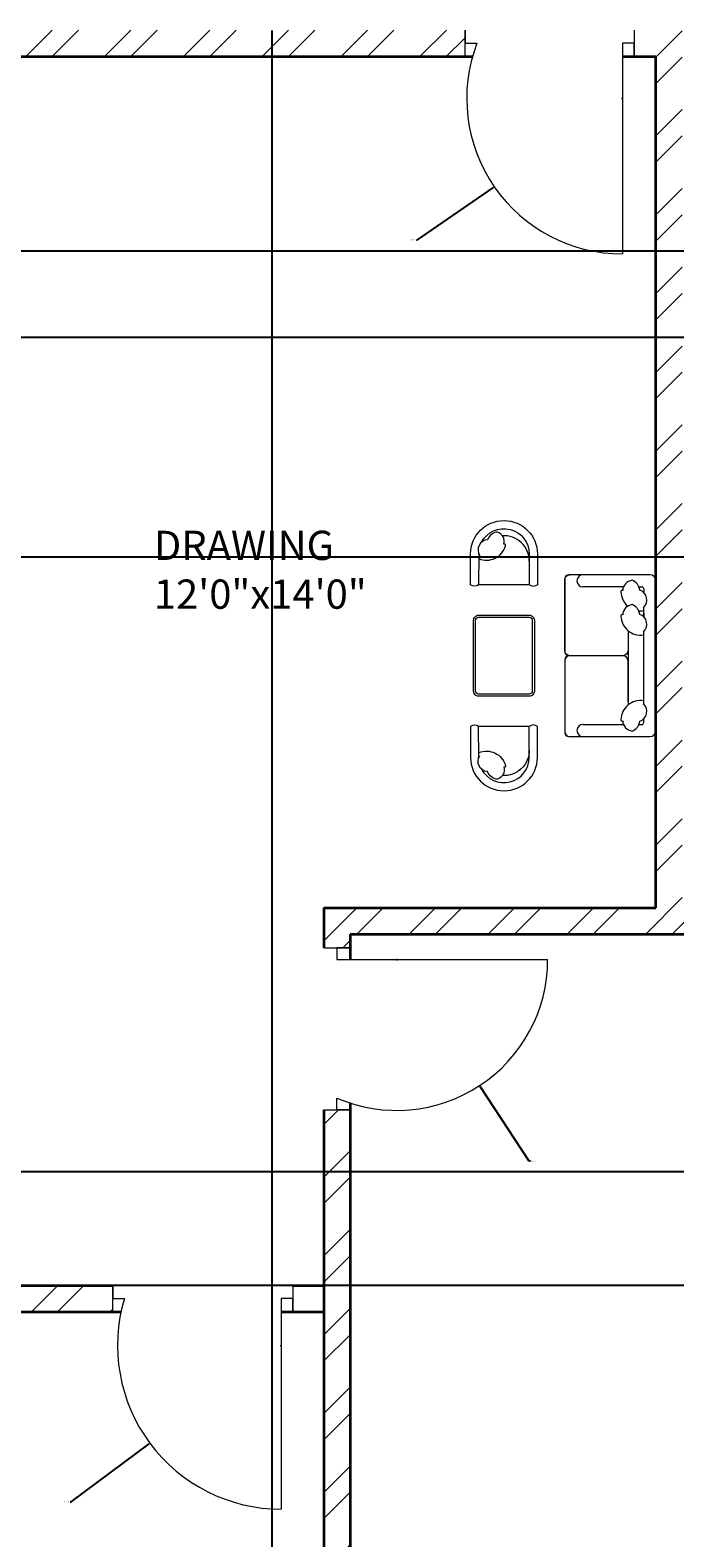
# Model space of a CAD drawing. Units: inches. Extents: x 2008 to 2657, y 1077 to 2165.
# Tile 4 of 16: x 2196 to 2306, y 1309 to 1567. Entities that reach past the tile are written whole.
import ezdxf

# ---------------------------------------------------------------- set-up
doc = ezdxf.new("R2010")
doc.units = ezdxf.units.IN
for name, color, linetype, lineweight in [('A-ANNO-DIMS', 2, 'Continuous', 18), ('A-AREA-IDEN', 4, 'Continuous', 18), ('A-DOOR', 11, 'Continuous', 18), ('A-FURN', 8, 'Continuous', 13), ('A-WALL', 7, 'Continuous', 35)]:
    doc.layers.add(name, color=color, linetype=linetype, lineweight=lineweight)
doc.layers.add('A-WALL-PATT', color=30, linetype='Continuous', lineweight=13, true_color=0xf8991e)
doc.styles.get("Standard").update_dxf_attribs({"font": 'arial.ttf'})
doc.dimstyles.get("Standard").update_dxf_attribs({"dimtxt": 0.18, "dimasz": 0.18, "dimexe": 0.18, "dimexo": 0.0625, "dimgap": 0.09, "dimtad": 0, "dimtih": 1, "dimtoh": 1, "dimdec": 4, "dimzin": 0, "dimdsep": 46, "dimtxsty": 'Standard', "dimcen": 0.09, "dimadec": 0, "dimazin": 0, "dimtfac": 1, "dimtdec": 4, "dimtofl": 0, "dimtmove": 0, "dimatfit": 3, "dimfxl": 1, "dimtolj": 1, "dimtzin": 0, "dimarcsym": 0})

# ---------------------------------------------------------------- blocks, each defined once
blk = doc.blocks.new('A$C1352')
at = {"color": 0}
for points in [[(0.003, 0.053), (0.003, 0.553, -0.414214), (0.053, 0.603), (0.753, 0.603, -0.414214), (0.803, 0.553), (0.803, 0.053, -0.414214), (0.753, 0.003), (0.053, 0.003, -0.414214)], [(0.023, 0.053), (0.023, 0.553, -0.414214), (0.053, 0.583), (0.753, 0.583, -0.414214), (0.783, 0.553), (0.783, 0.053, -0.414214), (0.753, 0.023), (0.053, 0.023, -0.414214)]]:
    blk.add_lwpolyline(points, format="xyb", close=True, dxfattribs=at)
blk = doc.blocks.new('LOUNGE-CHAIR')
blk.add_line((1.39, 5.54), (1.38, 0.26))
at = {"ltscale": 0.03}
blk.add_lwpolyline([(1.38, 0.26, -0.369229), (0, 0.27), (0, 5.54, -1), (11.42, 5.53), (11.42, 0.25, -0.369229), (10.03, 0.26)], format="xyb", close=True, dxfattribs=at)
blk.add_lwpolyline([(1.88, 7.54, -0.785087), (10.04, 5.53), (10.03, 0.26)], format="xyb")
for centre, radius, start, end in [((3.01, 6.23), 1.73, 92.9922, 214.1401), ((4.77, 7.34), 1.95, 94.9999, 161.3534), ((3.98, 7.61), 1.78, 346.6403, 69.4695), ((5.71, 4.32), 4.33, 359.9461, 93.658), ((5.71, 5.54), 4.33, 178.8536, 179.9461), ((2.75, 7.82), 3.35, 247.0143, 344.2857), ((5.79, 7.01), 0.207, 330.6238, 113.7423)]:
    blk.add_arc(centre, radius, start, end)
blk = doc.blocks.new('*D31')
at = {"layer": 'A-ANNO-DIMS', "color": 0, "lineweight": -2, "transparency": 16777216}
for p, q in [((2076.26, 1562.18), (2076.26, 1140.44)), ((2576.76, 1188.61), (2576.76, 1140.44)), ((2076.44, 1140.62), (2326.12, 1140.62)), ((2576.58, 1140.62), (2326.91, 1140.62))]:
    blk.add_line(p, q, dxfattribs=at)
at = {"layer": 'A-ANNO-DIMS', "color": 0, "transparency": 16777216}
for points in [[(2076.44, 1140.65), (2076.44, 1140.59), (2076.26, 1140.62)], [(2576.58, 1140.65), (2576.58, 1140.59), (2576.76, 1140.62)]]:
    blk.add_solid(points, dxfattribs=at)
at = {"layer": 'Defpoints', "color": 0, "transparency": 16777216}
for p in [(2076.26, 1562.24), (2576.76, 1188.67), (2576.76, 1140.62)]:
    blk.add_point(p, dxfattribs=at)
at = {"layer": 'A-ANNO-DIMS', "color": 0, "transparency": 16777216, "insert": (2326.51, 1140.62), "char_height": 0.18, "attachment_point": 5}
blk.add_mtext('\\A1;500.5', dxfattribs=at)
blk = doc.blocks.new('*D53')
at = {"layer": 'A-ANNO-DIMS', "color": 0, "lineweight": -2, "transparency": 16777216}
for p, q in [((2406.7, 1613.17), (2028.03, 1613.17)), ((2028.21, 1612.99), (2028.21, 1545.11)), ((2028.21, 1476.85), (2028.21, 1544.74)), ((2406.7, 1476.67), (2028.03, 1476.67))]:
    blk.add_line(p, q, dxfattribs=at)
at = {"layer": 'A-ANNO-DIMS', "color": 0, "transparency": 16777216}
for points in [[(2028.18, 1612.99), (2028.24, 1612.99), (2028.21, 1613.17)], [(2028.18, 1476.85), (2028.24, 1476.85), (2028.21, 1476.67)]]:
    blk.add_solid(points, dxfattribs=at)
at = {"layer": 'Defpoints', "color": 0, "transparency": 16777216}
for p in [(2406.76, 1613.17), (2028.21, 1476.67), (2406.76, 1476.67)]:
    blk.add_point(p, dxfattribs=at)
at = {"layer": 'A-ANNO-DIMS', "color": 0, "transparency": 16777216, "insert": (2028.21, 1544.92), "char_height": 0.18, "attachment_point": 5}
blk.add_mtext('\\A1;136.5', dxfattribs=at)
blk = doc.blocks.new('*D62')
at = {"layer": 'A-ANNO-DIMS', "color": 0, "lineweight": -2, "transparency": 16777216}
for p, q in [((2117.38, 1566.68), (2117.38, 1140.44)), ((2237.38, 1566.68), (2237.38, 1140.44)), ((2117.56, 1140.62), (2177.1, 1140.62)), ((2237.2, 1140.62), (2177.66, 1140.62))]:
    blk.add_line(p, q, dxfattribs=at)
at = {"layer": 'A-ANNO-DIMS', "color": 0, "transparency": 16777216}
for points in [[(2117.56, 1140.65), (2117.56, 1140.59), (2117.38, 1140.62)], [(2237.2, 1140.65), (2237.2, 1140.59), (2237.38, 1140.62)]]:
    blk.add_solid(points, dxfattribs=at)
at = {"layer": 'Defpoints', "color": 0, "transparency": 16777216}
for p in [(2117.38, 1566.74), (2237.38, 1566.74), (2237.38, 1140.62)]:
    blk.add_point(p, dxfattribs=at)
at = {"layer": 'A-ANNO-DIMS', "color": 0, "transparency": 16777216, "insert": (2177.38, 1140.62), "char_height": 0.18, "attachment_point": 5}
blk.add_mtext('\\A1;120', dxfattribs=at)
blk = doc.blocks.new('*D68')
at = {"layer": 'A-ANNO-DIMS', "color": 0, "lineweight": -2, "transparency": 16777216}
for p, q in [((2572.2, 1371.57), (2028.03, 1371.57)), ((2028.21, 1371.39), (2028.21, 1362.05)), ((2028.21, 1352.35), (2028.21, 1361.69)), ((2572.2, 1352.17), (2028.03, 1352.17))]:
    blk.add_line(p, q, dxfattribs=at)
at = {"layer": 'A-ANNO-DIMS', "color": 0, "transparency": 16777216}
for points in [[(2028.18, 1371.39), (2028.24, 1371.39), (2028.21, 1371.57)], [(2028.18, 1352.35), (2028.24, 1352.35), (2028.21, 1352.17)]]:
    blk.add_solid(points, dxfattribs=at)
at = {"layer": 'Defpoints', "color": 0, "transparency": 16777216}
for p in [(2028.21, 1371.57), (2572.26, 1371.57), (2572.26, 1352.17)]:
    blk.add_point(p, dxfattribs=at)
at = {"layer": 'A-ANNO-DIMS', "color": 0, "transparency": 16777216, "insert": (2028.21, 1361.87), "char_height": 0.18, "attachment_point": 5}
blk.add_mtext('\\A1;19.394', dxfattribs=at)
blk = doc.blocks.new('*D69')
at = {"layer": 'A-ANNO-DIMS', "color": 0, "lineweight": -2, "transparency": 16777216}
for p, q in [((2109.32, 1529), (2624.99, 1529)), ((2624.81, 1528.82), (2624.81, 1521.8)), ((2624.81, 1514.42), (2624.81, 1521.44)), ((2109.32, 1514.24), (2624.99, 1514.24))]:
    blk.add_line(p, q, dxfattribs=at)
at = {"layer": 'A-ANNO-DIMS', "color": 0, "transparency": 16777216}
for points in [[(2624.78, 1528.82), (2624.84, 1528.82), (2624.81, 1529)], [(2624.78, 1514.42), (2624.84, 1514.42), (2624.81, 1514.24)]]:
    blk.add_solid(points, dxfattribs=at)
at = {"layer": 'Defpoints', "color": 0, "transparency": 16777216}
for p in [(2109.26, 1529), (2624.81, 1529), (2109.26, 1514.24)]:
    blk.add_point(p, dxfattribs=at)
at = {"layer": 'A-ANNO-DIMS', "color": 0, "transparency": 16777216, "insert": (2624.81, 1521.62), "char_height": 0.18, "attachment_point": 5}
blk.add_mtext('\\A1;14.756', dxfattribs=at)
blk = doc.blocks.new('*D75')
at = {"layer": 'A-ANNO-DIMS', "color": 0, "lineweight": -2, "transparency": 16777216}
for p, q in [((2238.91, 1341.89), (2239.09, 1341.89)), ((2239, 1341.8), (2239, 1341.98)), ((2203.1, 1315.18), (2216.42, 1325.09)), ((2202.92, 1315.18), (2203.1, 1315.18))]:
    blk.add_line(p, q, dxfattribs=at)
at = {"layer": 'A-ANNO-DIMS', "color": 0, "transparency": 16777216}
blk.add_solid([(2216.4, 1325.11), (2216.43, 1325.06), (2216.56, 1325.2)], dxfattribs=at)
at = {"layer": 'Defpoints', "color": 0, "transparency": 16777216}
for p in [(2239, 1341.89), (2216.56, 1325.2)]:
    blk.add_point(p, dxfattribs=at)
at = {"layer": 'A-ANNO-DIMS', "color": 0, "transparency": 16777216, "insert": (2202.37, 1315.18), "char_height": 0.18, "attachment_point": 5}
blk.add_mtext('\\A1;R27.965', dxfattribs=at)
blk = doc.blocks.new('*D78')
at = {"layer": 'A-ANNO-DIMS', "color": 0, "lineweight": -2, "transparency": 16777216}
for p, q in [((2297.18, 1555.08), (2297.36, 1555.08)), ((2297.27, 1554.99), (2297.27, 1555.17)), ((2262.27, 1530.9), (2275.25, 1539.87)), ((2262.09, 1530.9), (2262.27, 1530.9))]:
    blk.add_line(p, q, dxfattribs=at)
at = {"layer": 'A-ANNO-DIMS', "color": 0, "transparency": 16777216}
blk.add_solid([(2275.23, 1539.89), (2275.26, 1539.84), (2275.39, 1539.97)], dxfattribs=at)
at = {"layer": 'Defpoints', "color": 0, "transparency": 16777216}
for p in [(2297.27, 1555.08), (2275.39, 1539.97)]:
    blk.add_point(p, dxfattribs=at)
at = {"layer": 'A-ANNO-DIMS', "color": 0, "transparency": 16777216, "insert": (2261.61, 1530.9), "char_height": 0.18, "attachment_point": 5}
blk.add_mtext('\\A1;R26.59', dxfattribs=at)
blk = doc.blocks.new('*D80')
at = {"layer": 'A-ANNO-DIMS', "color": 0, "lineweight": -2, "transparency": 16777216}
for p, q in [((2258.65, 1407.86), (2258.83, 1407.86)), ((2258.74, 1407.77), (2258.74, 1407.95)), ((2281.38, 1373.4), (2272.99, 1386.17)), ((2281.56, 1373.4), (2281.38, 1373.4))]:
    blk.add_line(p, q, dxfattribs=at)
at = {"layer": 'A-ANNO-DIMS', "color": 0, "transparency": 16777216}
blk.add_solid([(2273.02, 1386.19), (2272.97, 1386.16), (2272.89, 1386.32)], dxfattribs=at)
at = {"layer": 'Defpoints', "color": 0, "transparency": 16777216}
for p in [(2258.74, 1407.86), (2272.89, 1386.32)]:
    blk.add_point(p, dxfattribs=at)
at = {"layer": 'A-ANNO-DIMS', "color": 0, "transparency": 16777216, "insert": (2282.04, 1373.4), "char_height": 0.18, "attachment_point": 5}
blk.add_mtext('\\A1;R25.77', dxfattribs=at)

msp = doc.modelspace()

# ---------------------------------------------------------------- hatches: boundary and pattern name
at = {"layer": 'A-WALL-PATT'}
h = msp.add_hatch(dxfattribs=at)
h.set_pattern_fill('ANSI32', color=256)
h.paths.add_polyline_path([(2109.2619, 2094.6743), (2104.7619, 2094.6743), (2104.7619, 2072.1743), (2104.7619, 2021.6151), (2109.2619, 2021.6151), (2109.2619, 2055.6743), (2126.1387, 2055.6743), (2126.1387, 2057.9243), (2126.1387, 2060.1743), (2109.2619, 2060.1743)])
h.paths.add_polyline_path([(2223.2494, 2057.9243), (2223.2494, 2060.1743), (2186.1387, 2060.1743), (2186.1387, 2055.6743), (2223.2494, 2055.6743)])
h.paths.add_polyline_path([(2250.7619, 2072.1743), (2250.7619, 2090.1743), (2250.7619, 2094.6743), (2246.2619, 2094.6743), (2246.2619, 2060.1743), (2242.7242, 2060.1743), (2242.7242, 2055.6743), (2246.2619, 2055.6743), (2246.2619, 1899.6743), (2242.7458, 1899.6743), (2242.7458, 1897.4243), (2242.7458, 1895.1743), (2246.2619, 1895.1743), (2246.2619, 1878.8745), (2248.5119, 1878.8745), (2250.7619, 1878.8745), (2250.7619, 1991.1743), (2250.7619, 2025.6743), (2257.6798, 2025.6743), (2257.6798, 2027.9243), (2257.6798, 2030.1743), (2250.7619, 2030.1743)])
h.paths.add_polyline_path([(2411.2619, 2031.6743), (2409.0119, 2031.6743), (2406.7619, 2031.6743), (2406.7619, 2030.1743), (2322.7619, 2030.1743), (2322.7619, 2053.3443), (2318.2619, 2053.3443), (2318.2619, 2030.1743), (2305.6798, 2030.1743), (2305.6798, 2025.6743), (2318.2619, 2025.6743), (2322.7619, 2025.6743), (2406.7619, 2025.6743), (2406.7619, 1995.6743), (2406.7619, 1847.2677), (2250.7619, 1847.2677), (2250.7619, 1850.9902), (2248.5119, 1850.9902), (2246.2619, 1850.9902), (2246.2619, 1847.1743), (2246.2619, 1842.7677), (2303.0015, 1842.7677), (2303.0015, 1667.2413), (2298.4208, 1667.2413), (2298.4208, 1662.7413), (2303.0015, 1662.7413), (2303.0015, 1649.8758), (2307.5015, 1649.8758), (2307.5015, 1842.7677), (2406.7619, 1842.7677), (2411.2619, 1842.7677), (2411.2619, 1878.6743), (2415.8196, 1878.6743), (2415.8196, 1880.9243), (2415.8196, 1883.1743), (2411.2619, 1883.1743)])
h.paths.add_polyline_path([(2411.2619, 2094.6743), (2406.7619, 2094.6743), (2318.2619, 2094.6743), (2318.2619, 2077.3443), (2322.7619, 2077.3443), (2322.7619, 2090.1743), (2406.7619, 2090.1743), (2406.7619, 2072.1743), (2406.7619, 2067.6743), (2406.7619, 2052.7524), (2411.2619, 2052.7524), (2411.2619, 2055.6743), (2414.9888, 2055.6743), (2414.9888, 2057.9243), (2414.9888, 2060.1743), (2411.2619, 2060.1743), (2411.2619, 2072.1743)])
h.paths.add_polyline_path([(2576.7619, 2072.1743), (2576.7619, 2094.6743), (2572.2619, 2094.6743), (2572.2619, 2060.1743), (2525.8113, 2060.1743), (2525.8113, 2055.6743), (2572.2619, 2055.6743), (2572.2619, 1994.289), (2576.7619, 1994.289)])
h.paths.add_polyline_path([(2465.8113, 2060.1743), (2436.2802, 2060.1743), (2436.2802, 2055.6743), (2465.8113, 2055.6743), (2465.8113, 2057.9243)])
h.paths.add_polyline_path([(2576.7619, 1934.289), (2574.5119, 1934.289), (2572.2619, 1934.289), (2572.2619, 1883.1743), (2447.7027, 1883.1743), (2447.7027, 1878.6743), (2459.7619, 1878.6743), (2459.7619, 1830.4982), (2464.2619, 1830.4982), (2464.2619, 1878.6743), (2572.2619, 1878.6743), (2572.2619, 1868.4883), (2576.7619, 1868.4883)])
h.paths.add_polyline_path([(2576.7619, 1832.4883), (2572.2619, 1832.4883), (2572.2619, 1806.6743), (2464.2619, 1806.6743), (2464.2619, 1809.6629), (2459.7619, 1809.6629), (2459.7619, 1802.1743), (2483.7619, 1802.1743), (2483.7619, 1778.1743), (2488.2619, 1778.1743), (2488.2619, 1802.1743), (2572.2619, 1802.1743), (2572.2619, 1793.6101), (2576.7619, 1793.6101)])
h.paths.add_polyline_path([(2576.7619, 1769.6101), (2572.2619, 1769.6101), (2572.2619, 1754.1743), (2488.2619, 1754.1743), (2488.2619, 1757.2675), (2486.0119, 1757.2675), (2483.7619, 1757.2675), (2483.7619, 1754.1743), (2447.4528, 1754.1743), (2447.4528, 1749.6743), (2483.7619, 1749.6743), (2572.2619, 1749.6743), (2572.2619, 1715.1837), (2576.7619, 1715.1837)])
h.paths.add_polyline_path([(2576.7619, 1655.1837), (2572.2619, 1655.1837), (2572.2619, 1617.6743), (2411.2619, 1617.6743), (2411.2619, 1749.6743), (2414.2827, 1749.6743), (2414.2827, 1754.1743), (2406.7619, 1754.1743), (2406.7619, 1749.6743), (2406.7619, 1617.6743), (2307.5015, 1617.6743), (2307.5015, 1621.0007), (2305.2515, 1621.0007), (2303.0015, 1621.0007), (2303.0015, 1609.6944), (2307.5015, 1609.6944), (2307.5015, 1613.1743), (2406.7619, 1613.1743), (2406.7619, 1476.6743), (2415.532, 1476.6743), (2415.532, 1478.9243), (2415.532, 1481.1743), (2411.2619, 1481.1743), (2411.2619, 1613.1743), (2572.2619, 1613.1743), (2572.2619, 1584.6086), (2576.7619, 1584.6086)])
h.paths.add_polyline_path([(2576.7619, 1524.6086), (2572.2619, 1524.6086), (2572.2619, 1481.1743), (2483.7619, 1481.1743), (2447.5119, 1481.1743), (2447.5119, 1476.6743), (2483.7619, 1476.6743), (2483.7619, 1473.5051), (2488.2619, 1473.5051), (2488.2619, 1476.6743), (2572.2619, 1476.6743), (2572.2619, 1469.5488), (2576.7619, 1469.5488)])
h.paths.add_polyline_path([(2576.7619, 1445.5488), (2572.2619, 1445.5488), (2572.2619, 1428.6743), (2488.2619, 1428.6743), (2488.2619, 1455.6743), (2486.0119, 1455.6743), (2483.7619, 1455.6743), (2483.7619, 1428.6743), (2459.7619, 1428.6743), (2459.7619, 1422.1519), (2464.2619, 1422.1519), (2464.2619, 1424.1743), (2572.2619, 1424.1743), (2572.2619, 1407.5685), (2576.7619, 1407.5685)])
h.paths.add_polyline_path([(2576.7619, 1371.5685), (2572.2619, 1371.5685), (2572.2619, 1352.1743), (2464.2619, 1352.1743), (2464.2619, 1403.1384), (2462.0119, 1403.1384), (2459.7619, 1403.1384), (2459.7619, 1352.1743), (2446.3194, 1352.1743), (2446.3194, 1347.6743), (2572.2619, 1347.6743), (2572.2619, 1321.0291), (2576.7619, 1321.0291)])
h.paths.add_polyline_path([(2462.703, 1227.6743), (2436.0298, 1227.6743), (2436.0298, 1225.4243), (2436.0298, 1223.1743), (2462.703, 1223.1743), (2462.703, 1225.4243)])
h.paths.add_polyline_path([(2576.7619, 1261.0291), (2574.5119, 1261.0291), (2572.2619, 1261.0291), (2572.2619, 1227.6743), (2522.703, 1227.6743), (2522.703, 1223.1743), (2572.2619, 1223.1743), (2572.2619, 1188.6743), (2576.7619, 1188.6743), (2576.7619, 1193.1743), (2576.7619, 1223.1743)])
h.paths.add_polyline_path([(2414.2823, 1227.6743), (2411.2619, 1227.6743), (2411.2619, 1267.1779), (2409.0119, 1267.1779), (2406.7619, 1267.1779), (2406.7619, 1227.6743), (2322.7619, 1227.6743), (2322.7619, 1244.3623), (2318.2619, 1244.3623), (2318.2619, 1223.1743), (2406.7619, 1223.1743), (2406.7619, 1193.1743), (2406.7619, 1188.6743), (2411.2619, 1188.6743), (2411.2619, 1193.1743), (2411.2619, 1223.1743), (2414.2823, 1223.1743)])
h.paths.add_polyline_path([(2411.2619, 1347.6743), (2414.702, 1347.6743), (2414.702, 1349.9243), (2414.702, 1352.1743), (2411.2619, 1352.1743), (2411.2619, 1416.7413), (2307.5015, 1416.7413), (2307.5015, 1579.8489), (2305.2515, 1579.8489), (2303.0015, 1579.8489), (2303.0015, 1566.7413), (2299.2719, 1566.7413), (2299.2719, 1562.2413), (2303.0015, 1562.2413), (2303.0015, 1416.7413), (2246.2619, 1416.7413), (2246.2619, 1409.8616), (2250.7619, 1409.8616), (2250.7619, 1412.2413), (2406.7619, 1412.2413), (2406.7619, 1292.1743), (2304.9703, 1292.1743), (2304.9703, 1287.6743), (2318.2619, 1287.6743), (2318.2619, 1268.3623), (2322.7619, 1268.3623), (2322.7619, 1287.6743), (2406.7619, 1287.6743), (2406.7619, 1285.4748), (2411.2619, 1285.4748)])
h.paths.add_polyline_path([(2109.2619, 1262.7482), (2104.7619, 1262.7482), (2104.7619, 1223.1743), (2104.7619, 1193.1743), (2104.7619, 1188.6743), (2109.2619, 1188.6743), (2109.2619, 1223.1743), (2126.7928, 1223.1743), (2126.7928, 1225.4243), (2126.7928, 1227.6743), (2109.2619, 1227.6743)])
h.paths.add_polyline_path([(2222.3268, 1227.6743), (2186.7928, 1227.6743), (2186.7928, 1223.1743), (2222.3268, 1223.1743)])
h.paths.add_polyline_path([(2250.7619, 1287.6743), (2256.9703, 1287.6743), (2256.9703, 1289.9243), (2256.9703, 1292.1743), (2250.7619, 1292.1743), (2250.7619, 1382.2078), (2248.5119, 1382.2078), (2246.2619, 1382.2078), (2246.2619, 1347.6743), (2246.2619, 1227.6743), (2242.6068, 1227.6743), (2242.6068, 1223.1743), (2246.2619, 1223.1743), (2246.2619, 1188.6743), (2250.7619, 1188.6743), (2250.7619, 1193.1743), (2250.7619, 1227.6743)])
h.paths.add_polyline_path([(2133.2619, 1349.9243), (2133.2619, 1352.1743), (2109.2619, 1352.1743), (2109.2619, 1375.2826), (2104.7619, 1375.2826), (2104.7619, 1322.7482), (2109.2619, 1322.7482), (2109.2619, 1347.6743), (2133.2619, 1347.6743)])
h.paths.add_polyline_path([(2210.2105, 1352.1743), (2161.7619, 1352.1743), (2161.7619, 1412.2413), (2185.7619, 1412.2413), (2185.7619, 1420.1851), (2183.5119, 1420.1851), (2181.2619, 1420.1851), (2181.2619, 1416.7413), (2109.2619, 1416.7413), (2109.2619, 1452.4006), (2104.7619, 1452.4006), (2104.7619, 1399.2826), (2109.2619, 1399.2826), (2109.2619, 1412.2413), (2157.2619, 1412.2413), (2157.2619, 1352.1743), (2154.3383, 1352.1743), (2154.3383, 1347.6743), (2210.2105, 1347.6743)])
h.paths.add_polyline_path([(2185.7619, 1514.2413), (2161.7619, 1514.2413), (2161.7619, 1518.1307), (2159.5119, 1518.1307), (2157.2619, 1518.1307), (2157.2619, 1514.2413), (2109.2619, 1514.2413), (2109.2619, 1528.997), (2107.0119, 1528.997), (2104.7619, 1528.997), (2104.7619, 1488.4006), (2109.2619, 1488.4006), (2109.2619, 1509.7413), (2181.2619, 1509.7413), (2181.2619, 1441.2042), (2185.7619, 1441.2042)])
h.paths.add_polyline_path([(2270.4025, 1566.7413), (2109.2619, 1566.7413), (2080.7619, 1566.7413), (2080.7619, 1586.5643), (2076.2619, 1586.5643), (2076.2619, 1562.2413), (2080.7619, 1562.2413), (2104.7619, 1562.2413), (2104.7619, 1552.997), (2109.2619, 1552.997), (2109.2619, 1562.2413), (2157.2619, 1562.2413), (2157.2619, 1538.2413), (2161.7619, 1538.2413), (2161.7619, 1562.2413), (2205.2619, 1562.2413), (2270.4025, 1562.2413)])
h.paths.add_polyline_path([(2131.6813, 1897.4243), (2131.6813, 1899.6743), (2109.2619, 1899.6743), (2109.2619, 1961.6151), (2104.7619, 1961.6151), (2104.7619, 1886.8042), (2109.2619, 1886.8042), (2109.2619, 1895.1743), (2131.6813, 1895.1743)])
h.paths.add_polyline_path([(2185.7619, 1847.1743), (2161.7619, 1847.1743), (2161.7619, 1895.1743), (2185.7619, 1895.1743), (2211.543, 1895.1743), (2211.543, 1897.4243), (2211.543, 1899.6743), (2154.0916, 1899.6743), (2154.0916, 1897.4243), (2154.0916, 1895.1743), (2157.2619, 1895.1743), (2157.2619, 1847.1743), (2109.2619, 1847.1743), (2109.2619, 1862.8042), (2104.7619, 1862.8042), (2104.7619, 1821.243), (2109.2619, 1821.243), (2109.2619, 1842.6743), (2181.2619, 1842.6743), (2181.2619, 1840.6763), (2185.7619, 1840.6763)])
h.paths.add_polyline_path([(2109.2619, 1785.243), (2104.7619, 1785.243), (2104.7619, 1715.4691), (2109.2619, 1715.4691), (2109.2619, 1730.8423), (2157.2619, 1730.8423), (2157.2619, 1727.6404), (2161.7619, 1727.6404), (2161.7619, 1730.8423), (2185.7619, 1730.8423), (2185.7619, 1822.1438), (2183.5119, 1822.1438), (2181.2619, 1822.1438), (2181.2619, 1735.3423), (2109.2619, 1735.3423)])
h.paths.add_polyline_path([(2109.2619, 1691.4691), (2104.7619, 1691.4691), (2104.7619, 1667.2413), (2076.2619, 1667.2413), (2076.2619, 1646.5643), (2080.7619, 1646.5643), (2080.7619, 1662.7413), (2109.2619, 1662.7413), (2271.4941, 1662.7413), (2271.4941, 1664.9913), (2271.4941, 1667.2413), (2181.2619, 1667.2413), (2161.7619, 1667.2413), (2161.7619, 1708.3752), (2159.5119, 1708.3752), (2157.2619, 1708.3752), (2157.2619, 1667.2413), (2109.2619, 1667.2413)])
h.paths.add_polyline_path([(2233.1467, 1747.4973), (2270.0737, 1747.4973), (2270.0737, 1766.1547), (2233.1467, 1766.1547)], flags=9)

# ---------------------------------------------------------------- linework, layer by layer
at = {"layer": 'A-DOOR'}
for p, q in [((2270.4025, 1562.2413), (2270.4025, 1566.7413)), ((2270.4025, 1566.7413), (2270.4025, 1564.4913)), ((2270.4025, 1564.4913), (2272.4025, 1564.4913)), ((2299.2719, 1564.4913), (2297.2719, 1564.4913)), ((2297.2719, 1564.4913), (2297.2719, 1528.4913)), ((2299.2719, 1566.7413), (2299.2719, 1562.2413)), ((2299.2719, 1562.2413), (2299.2719, 1564.4913)), ((2246.2619, 1409.8616), (2250.7619, 1409.8616)), ((2250.7619, 1409.8616), (2248.5119, 1409.8616)), ((2248.5119, 1409.8616), (2248.5119, 1407.8616)), ((2248.5119, 1407.8616), (2284.5119, 1407.8616)), ((2248.5119, 1382.2078), (2248.5119, 1384.2078)), ((2246.2619, 1382.2078), (2250.7619, 1382.2078)), ((2250.7619, 1382.2078), (2248.5119, 1382.2078)), ((2210.2105, 1347.6743), (2210.2105, 1352.1743)), ((2210.2105, 1352.1743), (2210.2105, 1349.9243)), ((2240.9956, 1352.1743), (2240.9956, 1347.6743)), ((2210.2105, 1349.9243), (2212.2105, 1349.9243)), ((2240.9956, 1349.9243), (2238.9956, 1349.9243)), ((2238.9956, 1349.9243), (2238.9956, 1313.9243)), ((2240.9956, 1347.6743), (2240.9956, 1349.9243))]:
    msp.add_line(p, q, dxfattribs=at)
for centre, radius, start, end in [((2297.2719, 1555.0814), 26.5901, 159.274584, 270), ((2258.7411, 1407.8616), 25.7708, 246.613663, 0), ((2238.9956, 1341.8888), 27.9645, 163.300855, 270)]:
    msp.add_arc(centre, radius, start, end, dxfattribs=at)
at = {"layer": 'A-FURN'}
for p, q in [((2297.4708, 1471.5852), (2290.5437, 1471.5852)), ((2300.0974, 1471.5852), (2300.5792, 1471.5852)), ((2300.9252, 1471.2391), (2300.9252, 1470.6025)), ((2300.9252, 1466.4484), (2300.9252, 1468.1043)), ((2300.9252, 1467.085), (2300.9252, 1466.4484)), ((2300.9252, 1451.5346), (2300.9252, 1463.9502)), ((2300.9252, 1448.3998), (2300.9252, 1449.0364)), ((2290.5437, 1448.0538), (2297.4708, 1448.0538)), ((2300.0974, 1448.0538), (2300.5792, 1448.0538))]:
    msp.add_line(p, q, dxfattribs=at)
at = {"layer": 'A-FURN', "ltscale": 0.03}
msp.add_lwpolyline([(2288.1214, 1459.811, 0.41421356), (2287.4293, 1459.1189), (2287.4293, 1446.6696, 0.41421356), (2288.1214, 1445.9775), (2301.9634, 1445.9775, 0.41421356), (2303.0015, 1447.0156), (2303.0015, 1472.6233, 0.41421356), (2301.9634, 1473.6615), (2288.1214, 1473.6615, 0.41421356), (2287.4293, 1472.9694), (2287.4293, 1460.5201, 0.41421356), (2288.1214, 1459.828)], format="xyb", dxfattribs=at)
at = {"layer": 'A-FURN'}
for points in [[(2298.2433, 1464.089), (2298.2433, 1460.6846, -0.41421356), (2297.3782, 1459.8195), (2288.2944, 1459.8195, -0.41421356), (2287.4293, 1460.6846), (2287.4293, 1472.7964, -0.41421356), (2288.2944, 1473.6615)], [(2298.2433, 1451.985), (2298.2433, 1458.9544, 0.41421356), (2297.3782, 1459.8195), (2288.2944, 1459.8195, 0.41421356), (2287.4293, 1458.9544), (2287.4293, 1446.8426, 0.41421356), (2288.2944, 1445.9775)]]:
    msp.add_lwpolyline(points, format="xyb", dxfattribs=at)
msp.add_lwpolyline([(2298.2433, 1464.089), (2298.2433, 1451.3958)], dxfattribs=at)
for centre, radius, start, end in [((2290.5437, 1472.6233), 1.0382, 90, 180), ((2290.5437, 1472.6233), 1.0382, 180, 270), ((2299.125, 1470.9329), 1.7781, 96.427858, 179.256998), ((2298.2873, 1470.8559), 1.9514, 4.543938, 70.89739), ((2300.5792, 1471.2391), 0.3461, 0, 90), ((2300.5792, 1471.2391), 0.3461, 0, 90), ((2297.22, 1470.7925), 0.207, 52.154994, 195.27353), ((2300.3687, 1470.8322), 3.3497, 181.611631, 229.375991), ((2299.723, 1469.3534), 1.7337, 311.757236, 72.905096), ((2297.22, 1466.6384), 0.207, 52.154994, 195.27353), ((2300.3687, 1466.6781), 3.3497, 181.611631, 278.88305), ((2299.125, 1466.7788), 1.7781, 96.427858, 179.256998), ((2298.2873, 1466.7017), 1.9514, 4.543938, 70.89739), ((2300.3687, 1470.8322), 3.3497, 264.880983, 278.88305), ((2299.723, 1465.1993), 1.7337, 311.757236, 72.905096), ((2300.3687, 1448.8067), 3.3497, 81.11695, 178.388369), ((2299.723, 1450.2855), 1.7337, 287.094904, 48.242764), ((2297.22, 1448.8464), 0.207, 164.72647, 307.845006), ((2299.125, 1448.706), 1.7781, 180.743002, 263.572142), ((2298.2873, 1448.7831), 1.9514, 289.10261, 355.456062), ((2300.5792, 1448.3998), 0.3461, 270, 0), ((2290.5437, 1447.0156), 1.0382, 90, 180), ((2290.5437, 1447.0156), 1.0382, 180, 270)]:
    msp.add_arc(centre, radius, start, end, dxfattribs=at)
at = {"layer": 'A-WALL'}
for p, q in [((2161.7619, 1562.2413), (2271.6639, 1562.2413)), ((2161.7619, 1562.2413), (2205.2619, 1562.2413)), ((2297.2719, 1562.2413), (2303.0015, 1562.2413)), ((2303.0015, 1416.7413), (2303.0015, 1562.2413)), ((2246.2619, 1416.7413), (2303.0015, 1416.7413)), ((2246.2619, 1416.7413), (2246.2619, 1409.8616)), ((2250.7619, 1412.2413), (2406.7619, 1412.2413)), ((2250.7619, 1412.2413), (2250.7619, 1407.8616)), ((2246.2619, 1382.2078), (2246.2619, 1347.6743)), ((2250.7619, 1383.3571), (2250.7619, 1292.1743)), ((2161.7619, 1352.1743), (2210.2105, 1352.1743)), ((2240.9956, 1352.1743), (2246.2619, 1352.1743)), ((2154.3383, 1347.6743), (2211.6361, 1347.6743)), ((2238.9956, 1347.6743), (2246.2619, 1347.6743)), ((2246.2619, 1347.6743), (2246.2619, 1227.6743))]:
    msp.add_line(p, q, dxfattribs=at)

# ---------------------------------------------------------------- block references
at = {"layer": 'A-FURN'}
msp.add_blockref('LOUNGE-CHAIR', (2271.3384, 1471.6712), dxfattribs=at)
at = {"layer": 'A-FURN', "ltscale": 0.03, "xscale": 17.30251319894821, "yscale": 17.30251319894821, "zscale": 17.30251319894821, "rotation": 270}
msp.add_blockref('A$C1352', (2271.8052, 1466.787), dxfattribs=at)
at = {"layer": 'A-FURN', "extrusion": (0, 0, -1), "zscale": -1, "rotation": 180}
msp.add_blockref('LOUNGE-CHAIR', (-2271.3384, 1447.9677), dxfattribs=at)

# ---------------------------------------------------------------- texts
at = {"layer": 'A-AREA-IDEN', "insert": (2217.2348, 1481.1743), "char_height": 5, "attachment_point": 1}
msp.add_mtext_dynamic_manual_height_columns('DRAWING\\P12\'0"x14\'0"', width=189.527125, gutter_width=12.5, heights=[0], dxfattribs=at)

# ---------------------------------------------------------------- dimensions: what is measured, and where the dimension line sits
at = {"layer": 'A-ANNO-DIMS'}
for base, p1, p2, override, picture, middle in [((2028.2119, 1476.6743), (2406.7619, 1613.1743), (2406.7619, 1476.6743), {"dimdec": 1, "dimlfac": 1, "dimrnd": 0, "dimzin": 0, "dimdsep": 46, "dimlunit": 2}, '*D53', (2028.2119, 1544.9243)), ((2624.8119, 1528.997), (2109.2619, 1514.2413), (2109.2619, 1528.997), {"dimdec": 3, "dimlfac": 1, "dimrnd": 0, "dimzin": 0, "dimdsep": 46, "dimlunit": 2}, '*D69', (2624.8119, 1521.6192)), ((2028.2119, 1371.5685), (2572.2619, 1352.1743), (2572.2619, 1371.5685), {"dimdec": 3, "dimlfac": 1, "dimrnd": 0, "dimzin": 0, "dimdsep": 46, "dimlunit": 2}, '*D68', (2028.2119, 1361.8714))]:
    dim = msp.add_linear_dim(base=base, p1=p1, p2=p2, angle=90, dimstyle='Standard', override=override, dxfattribs=at)
    dim.commit()
    dim.dimension.update_dxf_attribs({"geometry": picture, "text_midpoint": middle})
for base, p1, p2, override, picture, middle in [((2237.3789, 1140.6243), (2117.3789, 1566.7413), (2237.3789, 1566.7413), {"dimdec": 0, "dimlfac": 1, "dimrnd": 0, "dimzin": 0, "dimdsep": 46, "dimlunit": 2}, '*D62', (2177.3789, 1140.6243)), ((2576.7619, 1140.6243), (2076.2619, 1562.2413), (2576.7619, 1188.6743), {"dimdec": 1, "dimlfac": 1, "dimrnd": 0, "dimzin": 0, "dimdsep": 46, "dimlunit": 2}, '*D31', (2326.5119, 1140.6243))]:
    dim = msp.add_linear_dim(base=base, p1=p1, p2=p2, dimstyle='Standard', override=override, dxfattribs=at)
    dim.commit()
    dim.dimension.update_dxf_attribs({"geometry": picture, "text_midpoint": middle})
for center, mpoint, override, picture, middle in [((2297.2719, 1555.0814), (2275.3944, 1539.9683), {"dimdec": 2, "dimlfac": 1, "dimrnd": 0, "dimzin": 0, "dimdsep": 46, "dimlunit": 2}, '*D78', (2261.6079, 1530.9004)), ((2258.7411, 1407.8616), (2272.8922, 1386.3237), {"dimdec": 2, "dimlfac": 1, "dimrnd": 0, "dimzin": 0, "dimdsep": 46, "dimlunit": 2}, '*D80', (2282.0427, 1373.4009)), ((2238.9956, 1341.8888), (2216.5599, 1325.1959), {"dimdec": 3, "dimlfac": 1, "dimrnd": 0, "dimzin": 0, "dimdsep": 46, "dimlunit": 2}, '*D75', (2202.3681, 1315.1802))]:
    dim = msp.add_radius_dim(center=center, mpoint=mpoint, dimstyle='Standard', override=override, dxfattribs=at)
    dim.commit()
    dim.dimension.update_dxf_attribs({"geometry": picture, "text_midpoint": middle, "dimtype": 164})

doc.saveas('drawing.dxf')
